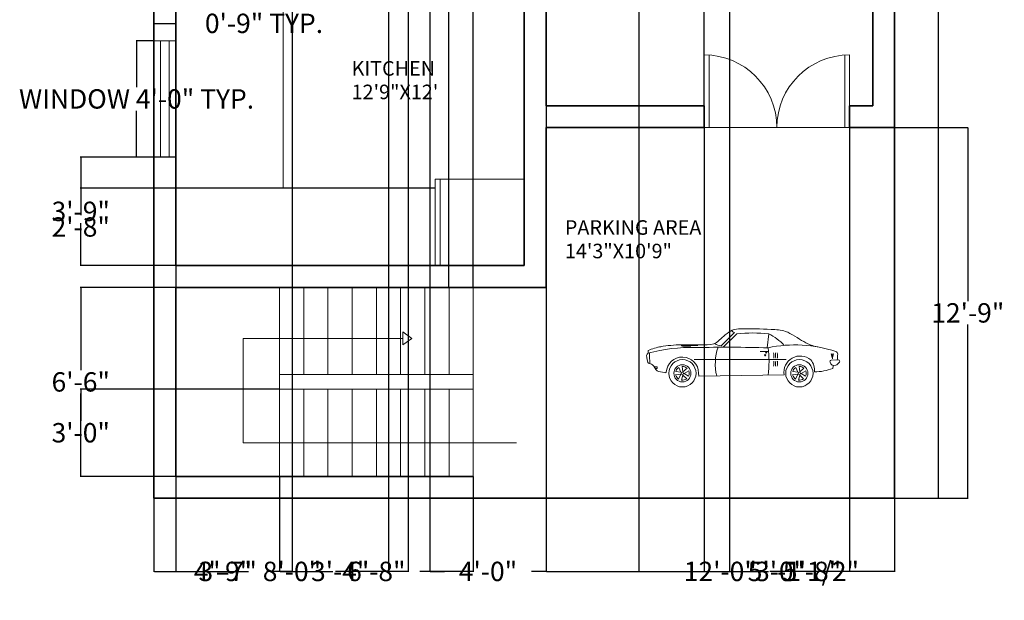
# Model space of a CAD drawing. Units: inches. Extents: x -69 to 405, y -4 to 680.
# Tile 1 of 3: x -34 to 372, y -4 to 236. Entities that reach past the tile are written whole.
import ezdxf

# ---------------------------------------------------------------- set-up
doc = ezdxf.new("R2010")
doc.units = ezdxf.units.IN
doc.header["$MEASUREMENT"] = 0
for name, color, linetype, lineweight in [('A-ANNO-DIMS', 4, 'Continuous', 18), ('A-AREA-IDEN', 4, 'Continuous', 18), ('A-EQPM-VEHI', 8, 'Continuous', 13), ('A-FLOR-CASE', 7, 'Continuous', 18), ('A-FLOR-STRS', 7, 'Continuous', 20), ('A-WALL', 7, 'Continuous', 35)]:
    doc.layers.add(name, color=color, linetype=linetype, lineweight=lineweight)
doc.layers.add('A-DOOR', color=2, linetype='Continuous', lineweight=18, true_color=0xf1eb1f)
doc.layers.add('A-GLAZ', color=85, linetype='Continuous', lineweight=18, true_color=0x58ba48)
doc.styles.get("Standard").update_dxf_attribs({"font": 'italic8.shx'})
doc.dimstyles.get("Standard").update_dxf_attribs({"dimtxt": 8, "dimasz": 0.18, "dimexe": 0.18, "dimexo": 0.0625, "dimgap": 0.09, "dimtad": 0, "dimtih": 1, "dimtoh": 1, "dimdec": 4, "dimzin": 0, "dimdsep": 46, "dimlunit": 3, "dimtxsty": 'Standard', "dimcen": 0.09, "dimadec": 0, "dimazin": 0, "dimtfac": 1, "dimtdec": 4, "dimtofl": 0, "dimtmove": 0, "dimatfit": 3, "dimfxl": 1, "dimtolj": 1, "dimtzin": 0, "dimarcsym": 0})

# ---------------------------------------------------------------- blocks, each defined once
blk = doc.blocks.new('*U2')
for p, q in [((72.93, 40.23), (85.8, 53.18)), ((75, 38.82), (88.08, 51.97)), ((119.39, 51.91), (117.92, 38.32)), ((50.13, 41.06), (34.31, 40.98)), ((43.26, 39.85), (35.15, 39.78)), ((35.3, 40.46), (50.13, 40.62)), ((111.09, 34.73), (118.48, 34.64)), ((7.45, 19.78), (9.74, 19.8)), ((46.65, 26.83), (136.29, 26.77)), ((179.3, 24.35), (180.25, 22.49)), ((180.37, 26.17), (187.51, 26.41)), ((182.62, 21.14), (184.91, 21.28)), ((186.68, 22.17), (188.51, 24.37)), ((9.76, 17.93), (8.53, 17.92)), ((10.37, 19.19), (10.38, 18.56)), ((50.87, 13.52), (50.91, 10.52))]:
    blk.add_line(p, q)
for points in [[(35.31, 39.93), (35.3, 40.27, 0.269532), (35.14, 40.54), (34.38, 40.96, 0.575383), (34.15, 40.83), (34.15, 40.49, 0.269532), (34.32, 40.22), (35.08, 39.79, 0.575383)], [(34.64, 20.05), (35.56, 14.97), (39.5, 18.31, 0.199906)], [(148.99, 20.05), (149.91, 14.97), (153.85, 18.31, 0.199906)], [(31.31, 7.72), (33.55, 12.37), (28.4, 11.99, 0.199906)], [(28.49, 15.1), (33.61, 14.4), (31.65, 19.18, 0.199906)], [(39.19, 8.12), (35.46, 11.69), (34.23, 6.67, 0.199906)], [(41.25, 15.74), (36.7, 13.3), (41.09, 10.58, 0.199906)], [(145.66, 7.72), (147.9, 12.37), (142.75, 11.99, 0.199906)], [(142.85, 15.1), (147.96, 14.4), (146.01, 19.18, 0.199906)], [(153.54, 8.12), (149.81, 11.69), (148.59, 6.67, 0.199906)], [(155.6, 15.74), (151.06, 13.3), (155.45, 10.58, 0.199906)]]:
    blk.add_lwpolyline(points, format="xyb", close=True)
for points in [[(181.58, 27.46), (181.53, 31.95), (180.48, 32.43)], [(181.58, 27.46), (181.53, 31.95), (182.57, 32.45)], [(50.91, 10.52), (134.38, 11.83)]]:
    blk.add_lwpolyline(points)
for centre, radius in [((115.89, 31.01), 0.619), ((34.98, 13.35), 13.35), ((34.98, 13.35), 8.35), ((149.33, 13.35), 13.35), ((149.33, 13.35), 8.35), ((34.98, 13.35), 1.25), ((149.33, 13.35), 1.25)]:
    blk.add_circle(centre, radius)
for centre, radius, start, end in [((114.6, 105.09), 59.37, 237.61027, 240.97846), ((103.45, -95), 147.78, 83.81633, 95.97054), ((95.51, 3.91), 53.61, 43.27479, 63.56652), ((42.18, -111.35), 149.91, 87.83928, 105.80965), ((20.53, -3.15), 43.06, 98.53035, 116.11198), ((80.1, -1364.13), 1402.96, 88.42296, 91.3179), ((73.29, 50.49), 10.26, 230.42401, 268.00854), ((118.31, 22.51), 51.16, 161.43071, 193.23633), ((145.17, -84.88), 125.99, 71.52833, 102.12419), ((79.16, 30.11), 76.3, 177.57734, 185.52052), ((34.98, 13.35), 15.9, 0.63732, 176.34123), ((25.66, 24.94), 94.01, 351.8279, 8.16738), ((45.64, 26.83), 78.76, 0.85201, 4.65562), ((47.43, 26.85), 78.76, 0.85201, 4.65562), ((49.23, 26.87), 78.76, 0.85201, 4.65562), ((150.1, 14.36), 15.92, 49.2263, 189.1528), ((216.26, 37.76), 36.17, 188.46832, 196.53145), ((146.68, 36.98), 36.17, 344.74319, 352.80633), ((184.3, 32.25), 2.49, 357.93203, 71.52833), ((116.55, 34.7), 70.29, 353.19423, 357.93203), ((9.75, 19.18), 0.623, 0.63732, 90.63732), ((45.64, 26.83), 78.76, 355.26443, 358.86328), ((47.43, 26.85), 78.76, 355.26443, 358.86328), ((49.23, 26.87), 78.76, 355.26443, 358.86328), ((149.4, 16.55), 14.84, 352.72855, 41.66131), ((180.41, 24.92), 1.25, 91.93898, 207.10902), ((182.47, 23.63), 2.49, 207.10902, 273.46767), ((114.25, 37.03), 70.29, 344.3985, 346.93849), ((184.76, 23.76), 2.49, 273.46767, 320.16835), ((187.55, 25.16), 1.25, 320.16835, 91.93898), ((9.76, 18.55), 0.623, 270.63732, 0.63732), ((162.47, 70.82), 56.18, 271.6865, 290.2774)]:
    blk.add_arc(centre, radius, start, end)
blk.add_ellipse((116.89, 33.59), major_axis=(-0.63, -0.007), ratio=0.610043)
for points, knots in [([(11.39, 38.92), (18.06, 40.19), (30.91, 42.01), (64.77, 40.11), (70.25, 44.91), (82.35, 56.38), (99.18, 57.3), (116.06, 56.35), (133.04, 55.87), (145.24, 49.87), (153.62, 43.8), (161.17, 40.68), (164.92, 39.73), (167.29, 39.15)], [18.629823, 18.629823, 18.629823, 18.629823, 19.527405, 20.700571, 21.107983, 21.608568, 21.92336, 23.151359, 23.716171, 23.908743, 24.77794, 24.943072, 25.187755, 25.187755, 25.187755, 25.187755]), ([(19.11, 14.36), (18.99, 14.21), (18.5, 13.81), (15.35, 15), (9.19, 13.94), (7.26, 22.22), (3.01, 22.66), (1.32, 23.61), (0.64, 26.92), (-0.96, 31.49), (1.54, 32.64), (1.5, 34.06), (1.49, 34.8), (1.49, 35.06), (1.52, 35.3), (1.58, 35.51)], [16.815853, 16.815853, 16.815853, 16.815853, 16.838212, 16.885395, 17.18439, 17.479846, 17.654423, 17.670693, 17.696923, 18.016358, 18.052739, 18.140805, 18.140805, 18.140805, 18.172382, 18.172382, 18.172382, 18.172382])]:
    blk.add_open_spline(points, degree=3, knots=knots)
blk = doc.blocks.new('*D5')
at = {"layer": 'A-ANNO-DIMS', "color": 0, "lineweight": -2, "transparency": 16777216}
for p, q in [((327.07, 638.28), (345.4, 638.28)), ((345.22, 638.1), (345.22, 343.14)), ((345.22, 38.46), (345.22, 333.43)), ((327.07, 38.28), (345.4, 38.28))]:
    blk.add_line(p, q, dxfattribs=at)
at = {"layer": 'A-ANNO-DIMS', "color": 0, "transparency": 16777216}
for points in [[(345.19, 638.1), (345.25, 638.1), (345.22, 638.28)], [(345.19, 38.46), (345.25, 38.46), (345.22, 38.28)]]:
    blk.add_solid(points, dxfattribs=at)
at = {"layer": 'Defpoints', "color": 0, "transparency": 16777216}
for p in [(327.01, 638.28), (327.01, 38.28), (345.22, 38.28)]:
    blk.add_point(p, dxfattribs=at)
at = {"layer": 'A-ANNO-DIMS', "color": 0, "transparency": 16777216, "insert": (345.22, 338.28), "char_height": 8, "attachment_point": 5}
blk.add_mtext("\\A1;50'", dxfattribs=at)
blk = doc.blocks.new('WIN-48IN')
for p, q in [((0, 48), (0, 0)), ((9, 48), (0, 48)), ((2.75, 48), (2.75, 0)), ((6.25, 48), (6.25, 0)), ((9, 0), (9, 48)), ((0, 0), (9, 0))]:
    blk.add_line(p, q)
blk = doc.blocks.new('*D16')
at = {"layer": 'A-ANNO-DIMS', "color": 0, "lineweight": -2, "transparency": 16777216}
for p, q in [((20.95, 227.12), (13.63, 227.12)), ((13.81, 226.94), (13.81, 207.97)), ((13.81, 179.3), (13.81, 198.26)), ((20.95, 179.12), (13.63, 179.12))]:
    blk.add_line(p, q, dxfattribs=at)
at = {"layer": 'A-ANNO-DIMS', "color": 0, "transparency": 16777216}
for points in [[(13.78, 226.94), (13.84, 226.94), (13.81, 227.12)], [(13.78, 179.3), (13.84, 179.3), (13.81, 179.12)]]:
    blk.add_solid(points, dxfattribs=at)
at = {"layer": 'Defpoints', "color": 0, "transparency": 16777216}
for p in [(13.81, 227.12), (21.01, 227.12), (21.01, 179.12)]:
    blk.add_point(p, dxfattribs=at)
at = {"layer": 'A-ANNO-DIMS', "color": 0, "transparency": 16777216, "insert": (13.81, 203.12), "char_height": 8, "attachment_point": 5}
blk.add_mtext('\\A1;WINDOW 4\'-0" TYP.', dxfattribs=at)
blk = doc.blocks.new('*D17')
at = {"layer": 'A-ANNO-DIMS', "color": 0, "lineweight": -2, "transparency": 16777216}
for p, q in [((21.01, 227.18), (21.01, 234.5)), ((21.19, 234.32), (29.83, 234.32)), ((30.01, 227.18), (30.01, 234.5)), ((30.01, 234.32), (30.19, 234.32))]:
    blk.add_line(p, q, dxfattribs=at)
at = {"layer": 'A-ANNO-DIMS', "color": 0, "transparency": 16777216}
for points in [[(21.19, 234.35), (21.19, 234.29), (21.01, 234.32)], [(29.83, 234.35), (29.83, 234.29), (30.01, 234.32)]]:
    blk.add_solid(points, dxfattribs=at)
at = {"layer": 'Defpoints', "color": 0, "transparency": 16777216}
for p in [(30.01, 234.32), (21.01, 227.12), (30.01, 227.12)]:
    blk.add_point(p, dxfattribs=at)
at = {"layer": 'A-ANNO-DIMS', "color": 0, "transparency": 16777216, "insert": (66.47, 234.32), "char_height": 8, "attachment_point": 5}
blk.add_mtext('\\A1;0\'-9" TYP.', dxfattribs=at)
blk = doc.blocks.new('*D24')
at = {"layer": 'A-ANNO-DIMS', "color": 0, "lineweight": -2, "transparency": 16777216}
for p, q in [((30.01, 47.22), (30.01, 7.85)), ((72.9, 47.22), (72.9, 7.85)), ((30.19, 8.03), (33.65, 8.03)), ((72.72, 8.03), (69.26, 8.03))]:
    blk.add_line(p, q, dxfattribs=at)
at = {"layer": 'A-ANNO-DIMS', "color": 0, "transparency": 16777216}
for points in [[(30.19, 8.06), (30.19, 8), (30.01, 8.03)], [(72.72, 8.06), (72.72, 8), (72.9, 8.03)]]:
    blk.add_solid(points, dxfattribs=at)
at = {"layer": 'Defpoints', "color": 0, "transparency": 16777216}
for p in [(30.01, 47.28), (72.9, 47.28), (72.9, 8.03)]:
    blk.add_point(p, dxfattribs=at)
at = {"layer": 'A-ANNO-DIMS', "color": 0, "transparency": 16777216, "insert": (51.46, 8.03), "char_height": 8, "attachment_point": 5}
blk.add_mtext('\\A1;3\'-7"', dxfattribs=at)
blk = doc.blocks.new('*D25')
at = {"layer": 'A-ANNO-DIMS', "color": 0, "lineweight": -2, "transparency": 16777216}
for p, q in [((72.9, 47.22), (72.9, 7.85)), ((152.9, 47.22), (152.9, 7.85)), ((73.08, 8.03), (94.91, 8.03)), ((152.72, 8.03), (130.9, 8.03))]:
    blk.add_line(p, q, dxfattribs=at)
at = {"layer": 'A-ANNO-DIMS', "color": 0, "transparency": 16777216}
for points in [[(73.08, 8.06), (73.08, 8), (72.9, 8.03)], [(152.72, 8.06), (152.72, 8), (152.9, 8.03)]]:
    blk.add_solid(points, dxfattribs=at)
at = {"layer": 'Defpoints', "color": 0, "transparency": 16777216}
for p in [(72.9, 47.28), (152.9, 47.28), (152.9, 8.03)]:
    blk.add_point(p, dxfattribs=at)
at = {"layer": 'A-ANNO-DIMS', "color": 0, "transparency": 16777216, "insert": (112.9, 8.03), "char_height": 8, "attachment_point": 5}
blk.add_mtext('\\A1;6\'-8"', dxfattribs=at)
blk = doc.blocks.new('*D26')
at = {"layer": 'A-ANNO-DIMS', "color": 0, "lineweight": -2, "transparency": 16777216}
for p, q in [((29.95, 125.28), (-9.42, 125.28)), ((-9.24, 125.1), (-9.24, 91.14)), ((-9.24, 47.46), (-9.24, 81.43)), ((29.95, 47.28), (-9.42, 47.28))]:
    blk.add_line(p, q, dxfattribs=at)
at = {"layer": 'A-ANNO-DIMS', "color": 0, "transparency": 16777216}
for points in [[(-9.27, 125.1), (-9.21, 125.1), (-9.24, 125.28)], [(-9.27, 47.46), (-9.21, 47.46), (-9.24, 47.28)]]:
    blk.add_solid(points, dxfattribs=at)
at = {"layer": 'Defpoints', "color": 0, "transparency": 16777216}
for p in [(-9.24, 125.28), (30.01, 125.28), (30.01, 47.28)]:
    blk.add_point(p, dxfattribs=at)
at = {"layer": 'A-ANNO-DIMS', "color": 0, "transparency": 16777216, "insert": (-9.24, 86.28), "char_height": 8, "attachment_point": 5}
blk.add_mtext('\\A1;6\'-6"', dxfattribs=at)
blk = doc.blocks.new('*D27')
at = {"layer": 'A-ANNO-DIMS', "color": 0, "lineweight": -2, "transparency": 16777216}
for p, q in [((72.84, 83.28), (-9.42, 83.28)), ((-9.24, 83.1), (-9.24, 70.14)), ((-9.24, 47.46), (-9.24, 60.43)), ((72.84, 47.28), (-9.42, 47.28))]:
    blk.add_line(p, q, dxfattribs=at)
at = {"layer": 'A-ANNO-DIMS', "color": 0, "transparency": 16777216}
for points in [[(-9.27, 83.1), (-9.21, 83.1), (-9.24, 83.28)], [(-9.27, 47.46), (-9.21, 47.46), (-9.24, 47.28)]]:
    blk.add_solid(points, dxfattribs=at)
at = {"layer": 'Defpoints', "color": 0, "transparency": 16777216}
for p in [(-9.24, 83.28), (72.9, 83.28), (72.9, 47.28)]:
    blk.add_point(p, dxfattribs=at)
at = {"layer": 'A-ANNO-DIMS', "color": 0, "transparency": 16777216, "insert": (-9.24, 65.28), "char_height": 8, "attachment_point": 5}
blk.add_mtext('\\A1;3\'-0"', dxfattribs=at)
blk = doc.blocks.new('*D28')
at = {"layer": 'A-ANNO-DIMS', "color": 0, "lineweight": -2, "transparency": 16777216}
for p, q in [((142.9, 125.35), (142.9, 668.71)), ((143.08, 668.53), (152.72, 668.53)), ((152.9, 125.35), (152.9, 668.71)), ((152.9, 668.53), (153.08, 668.53))]:
    blk.add_line(p, q, dxfattribs=at)
at = {"layer": 'A-ANNO-DIMS', "color": 0, "transparency": 16777216}
for points in [[(143.08, 668.56), (143.08, 668.5), (142.9, 668.53)], [(152.72, 668.56), (152.72, 668.5), (152.9, 668.53)]]:
    blk.add_solid(points, dxfattribs=at)
at = {"layer": 'Defpoints', "color": 0, "transparency": 16777216}
for p in [(152.9, 668.53), (142.9, 125.28), (152.9, 125.28)]:
    blk.add_point(p, dxfattribs=at)
at = {"layer": 'A-ANNO-DIMS', "color": 0, "transparency": 16777216, "insert": (173.75, 668.53), "char_height": 8, "attachment_point": 5}
blk.add_mtext('\\A1;0\'-10"', dxfattribs=at)
blk = doc.blocks.new('*D29')
at = {"layer": 'A-ANNO-DIMS', "color": 0, "lineweight": -2, "transparency": 16777216}
for p, q in [((183.01, 125.22), (183.01, 7.85)), ((327.01, 38.22), (327.01, 7.85)), ((183.19, 8.03), (234.54, 8.03)), ((326.83, 8.03), (275.48, 8.03))]:
    blk.add_line(p, q, dxfattribs=at)
at = {"layer": 'A-ANNO-DIMS', "color": 0, "transparency": 16777216}
for points in [[(183.19, 8.06), (183.19, 8), (183.01, 8.03)], [(326.83, 8.06), (326.83, 8), (327.01, 8.03)]]:
    blk.add_solid(points, dxfattribs=at)
at = {"layer": 'Defpoints', "color": 0, "transparency": 16777216}
for p in [(183.01, 125.28), (327.01, 38.28), (327.01, 8.03)]:
    blk.add_point(p, dxfattribs=at)
at = {"layer": 'A-ANNO-DIMS', "color": 0, "transparency": 16777216, "insert": (255.01, 8.03), "char_height": 8, "attachment_point": 5}
blk.add_mtext('\\A1;12\'-0"', dxfattribs=at)
blk = doc.blocks.new('*D30')
at = {"layer": 'A-ANNO-DIMS', "color": 0, "lineweight": -2, "transparency": 16777216}
for p, q in [((327.07, 191.28), (357.44, 191.28)), ((357.26, 191.1), (357.26, 119.64)), ((357.26, 38.46), (357.26, 109.93)), ((327.07, 38.28), (357.44, 38.28))]:
    blk.add_line(p, q, dxfattribs=at)
at = {"layer": 'A-ANNO-DIMS', "color": 0, "transparency": 16777216}
for points in [[(357.23, 191.1), (357.29, 191.1), (357.26, 191.28)], [(357.23, 38.46), (357.29, 38.46), (357.26, 38.28)]]:
    blk.add_solid(points, dxfattribs=at)
at = {"layer": 'Defpoints', "color": 0, "transparency": 16777216}
for p in [(327.01, 191.28), (327.01, 38.28), (357.26, 38.28)]:
    blk.add_point(p, dxfattribs=at)
at = {"layer": 'A-ANNO-DIMS', "color": 0, "transparency": 16777216, "insert": (357.26, 114.78), "char_height": 8, "attachment_point": 5}
blk.add_mtext('\\A1;12\'-9"', dxfattribs=at)
blk = doc.blocks.new('*D31')
at = {"layer": 'A-ANNO-DIMS', "color": 0, "lineweight": -2, "transparency": 16777216}
for p, q in [((248.38, 191.22), (248.38, 7.85)), ((308.38, 191.22), (308.38, 7.85)), ((248.56, 8.03), (260.39, 8.03)), ((308.2, 8.03), (296.38, 8.03))]:
    blk.add_line(p, q, dxfattribs=at)
at = {"layer": 'A-ANNO-DIMS', "color": 0, "transparency": 16777216}
for points in [[(248.56, 8.06), (248.56, 8), (248.38, 8.03)], [(308.2, 8.06), (308.2, 8), (308.38, 8.03)]]:
    blk.add_solid(points, dxfattribs=at)
at = {"layer": 'Defpoints', "color": 0, "transparency": 16777216}
for p in [(248.38, 191.28), (308.38, 191.28), (308.38, 8.03)]:
    blk.add_point(p, dxfattribs=at)
at = {"layer": 'A-ANNO-DIMS', "color": 0, "transparency": 16777216, "insert": (278.38, 8.03), "char_height": 8, "attachment_point": 5}
blk.add_mtext('\\A1;5\'-0"', dxfattribs=at)
blk = doc.blocks.new('*D32')
at = {"layer": 'A-ANNO-DIMS', "color": 0, "lineweight": -2, "transparency": 16777216}
for p, q in [((183.01, 200.35), (183.01, 668.71)), ((183.19, 668.53), (248.2, 668.53)), ((248.38, 200.35), (248.38, 668.71)), ((248.38, 668.53), (248.56, 668.53))]:
    blk.add_line(p, q, dxfattribs=at)
at = {"layer": 'A-ANNO-DIMS', "color": 0, "transparency": 16777216}
for points in [[(183.19, 668.56), (183.19, 668.5), (183.01, 668.53)], [(248.2, 668.56), (248.2, 668.5), (248.38, 668.53)]]:
    blk.add_solid(points, dxfattribs=at)
at = {"layer": 'Defpoints', "color": 0, "transparency": 16777216}
for p in [(248.38, 668.53), (183.01, 200.28), (248.38, 200.28)]:
    blk.add_point(p, dxfattribs=at)
at = {"layer": 'A-ANNO-DIMS', "color": 0, "transparency": 16777216, "insert": (281.8, 668.53), "char_height": 8, "attachment_point": 5}
blk.add_mtext('\\A1;5\'-5 1/2"', dxfattribs=at)
blk = doc.blocks.new('*D33')
at = {"layer": 'A-ANNO-DIMS', "color": 0, "lineweight": -2, "transparency": 16777216}
for p, q in [((30.01, 350.22), (30.01, 7.85)), ((126.01, 350.22), (126.01, 7.85)), ((30.19, 8.03), (60.01, 8.03)), ((125.83, 8.03), (96, 8.03))]:
    blk.add_line(p, q, dxfattribs=at)
at = {"layer": 'A-ANNO-DIMS', "color": 0, "transparency": 16777216}
for points in [[(30.19, 8.06), (30.19, 8), (30.01, 8.03)], [(125.83, 8.06), (125.83, 8), (126.01, 8.03)]]:
    blk.add_solid(points, dxfattribs=at)
at = {"layer": 'Defpoints', "color": 0, "transparency": 16777216}
for p in [(30.01, 350.28), (126.01, 350.28), (126.01, 8.03)]:
    blk.add_point(p, dxfattribs=at)
at = {"layer": 'A-ANNO-DIMS', "color": 0, "transparency": 16777216, "insert": (78.01, 8.03), "char_height": 8, "attachment_point": 5}
blk.add_mtext('\\A1;8\'-0"', dxfattribs=at)
blk = doc.blocks.new('*D40')
at = {"layer": 'A-ANNO-DIMS', "color": 0, "lineweight": -2, "transparency": 16777216}
for p, q in [((135.01, 407.22), (135.01, 7.85)), ((183.01, 407.22), (183.01, 7.85)), ((135.19, 8.03), (141.01, 8.03)), ((182.83, 8.03), (177, 8.03))]:
    blk.add_line(p, q, dxfattribs=at)
at = {"layer": 'A-ANNO-DIMS', "color": 0, "transparency": 16777216}
for points in [[(135.19, 8.06), (135.19, 8), (135.01, 8.03)], [(182.83, 8.06), (182.83, 8), (183.01, 8.03)]]:
    blk.add_solid(points, dxfattribs=at)
at = {"layer": 'Defpoints', "color": 0, "transparency": 16777216}
for p in [(135.01, 407.28), (183.01, 407.28), (183.01, 8.03)]:
    blk.add_point(p, dxfattribs=at)
at = {"layer": 'A-ANNO-DIMS', "color": 0, "transparency": 16777216, "insert": (159.01, 8.03), "char_height": 8, "attachment_point": 5}
blk.add_mtext('\\A1;4\'-0"', dxfattribs=at)
blk = doc.blocks.new('*D44')
at = {"layer": 'A-ANNO-DIMS', "color": 0, "lineweight": -2, "transparency": 16777216}
for p, q in [((21.01, 638.22), (21.01, 7.85)), ((78.06, 638.22), (78.06, 7.85)), ((21.19, 8.03), (31.54, 8.03)), ((77.88, 8.03), (67.53, 8.03))]:
    blk.add_line(p, q, dxfattribs=at)
at = {"layer": 'A-ANNO-DIMS', "color": 0, "transparency": 16777216}
for points in [[(21.19, 8.06), (21.19, 8), (21.01, 8.03)], [(77.88, 8.06), (77.88, 8), (78.06, 8.03)]]:
    blk.add_solid(points, dxfattribs=at)
at = {"layer": 'Defpoints', "color": 0, "transparency": 16777216}
for p in [(21.01, 638.28), (78.06, 638.28), (78.06, 8.03)]:
    blk.add_point(p, dxfattribs=at)
at = {"layer": 'A-ANNO-DIMS', "color": 0, "transparency": 16777216, "insert": (49.53, 8.03), "char_height": 8, "attachment_point": 5}
blk.add_mtext('\\A1;4\'-9"', dxfattribs=at)
blk = doc.blocks.new('*D45')
at = {"layer": 'A-ANNO-DIMS', "color": 0, "lineweight": -2, "transparency": 16777216}
for p, q in [((78.06, 638.22), (78.06, 7.85)), ((117.87, 638.22), (117.87, 7.85)), ((78.24, 8.03), (79.97, 8.03)), ((117.69, 8.03), (115.96, 8.03))]:
    blk.add_line(p, q, dxfattribs=at)
at = {"layer": 'A-ANNO-DIMS', "color": 0, "transparency": 16777216}
for points in [[(78.24, 8.06), (78.24, 8), (78.06, 8.03)], [(117.69, 8.06), (117.69, 8), (117.87, 8.03)]]:
    blk.add_solid(points, dxfattribs=at)
at = {"layer": 'Defpoints', "color": 0, "transparency": 16777216}
for p in [(78.06, 638.28), (117.87, 638.28), (117.87, 8.03)]:
    blk.add_point(p, dxfattribs=at)
at = {"layer": 'A-ANNO-DIMS', "color": 0, "transparency": 16777216, "insert": (97.96, 8.03), "char_height": 8, "attachment_point": 5}
blk.add_mtext('\\A1;3\'-4"', dxfattribs=at)
blk = doc.blocks.new('*D46')
at = {"layer": 'A-ANNO-DIMS', "color": 0, "lineweight": -2, "transparency": 16777216}
for p, q in [((221.33, 638.22), (221.33, 7.85)), ((258.77, 638.22), (258.77, 7.85)), ((221.51, 8.03), (258.59, 8.03)), ((258.77, 8.03), (258.95, 8.03))]:
    blk.add_line(p, q, dxfattribs=at)
at = {"layer": 'A-ANNO-DIMS', "color": 0, "transparency": 16777216}
for points in [[(221.51, 8.06), (221.51, 8), (221.33, 8.03)], [(258.59, 8.06), (258.59, 8), (258.77, 8.03)]]:
    blk.add_solid(points, dxfattribs=at)
at = {"layer": 'Defpoints', "color": 0, "transparency": 16777216}
for p in [(221.33, 638.28), (258.77, 638.28), (258.77, 8.03)]:
    blk.add_point(p, dxfattribs=at)
at = {"layer": 'A-ANNO-DIMS', "color": 0, "transparency": 16777216, "insert": (290.85, 8.03), "char_height": 8, "attachment_point": 5}
blk.add_mtext('\\A1;3\'-1 1/2"', dxfattribs=at)
blk = doc.blocks.new('*D47')
at = {"layer": 'A-ANNO-DIMS', "color": 0, "lineweight": -2, "transparency": 16777216}
for p, q in [((258.77, 638.22), (258.77, 7.85)), ((327.01, 638.22), (327.01, 7.85)), ((258.95, 8.03), (274.89, 8.03)), ((326.83, 8.03), (310.88, 8.03))]:
    blk.add_line(p, q, dxfattribs=at)
at = {"layer": 'A-ANNO-DIMS', "color": 0, "transparency": 16777216}
for points in [[(258.95, 8.06), (258.95, 8), (258.77, 8.03)], [(326.83, 8.06), (326.83, 8), (327.01, 8.03)]]:
    blk.add_solid(points, dxfattribs=at)
at = {"layer": 'Defpoints', "color": 0, "transparency": 16777216}
for p in [(258.77, 638.28), (327.01, 638.28), (327.01, 8.03)]:
    blk.add_point(p, dxfattribs=at)
at = {"layer": 'A-ANNO-DIMS', "color": 0, "transparency": 16777216, "insert": (292.89, 8.03), "char_height": 8, "attachment_point": 5}
blk.add_mtext('\\A1;5\'-8"', dxfattribs=at)
blk = doc.blocks.new('*D50')
at = {"layer": 'A-ANNO-DIMS', "color": 0, "lineweight": -2, "transparency": 16777216}
for p, q in [((29.95, 179.12), (-9.42, 179.12)), ((-9.24, 178.94), (-9.24, 161.55)), ((-9.24, 134.46), (-9.24, 151.85)), ((29.95, 134.28), (-9.42, 134.28))]:
    blk.add_line(p, q, dxfattribs=at)
at = {"layer": 'A-ANNO-DIMS', "color": 0, "transparency": 16777216}
for points in [[(-9.27, 178.94), (-9.21, 178.94), (-9.24, 179.12)], [(-9.27, 134.46), (-9.21, 134.46), (-9.24, 134.28)]]:
    blk.add_solid(points, dxfattribs=at)
at = {"layer": 'Defpoints', "color": 0, "transparency": 16777216}
for p in [(-9.24, 179.12), (30.01, 179.12), (30.01, 134.28)]:
    blk.add_point(p, dxfattribs=at)
at = {"layer": 'A-ANNO-DIMS', "color": 0, "transparency": 16777216, "insert": (-9.24, 156.7), "char_height": 8, "attachment_point": 5}
blk.add_mtext('\\A1;3\'-9"', dxfattribs=at)
blk = doc.blocks.new('*D64')
at = {"layer": 'A-ANNO-DIMS', "color": 0, "lineweight": -2, "transparency": 16777216}
for p, q in [((137.12, 166.22), (-9.42, 166.22)), ((-9.24, 166.04), (-9.24, 155.11)), ((-9.24, 134.46), (-9.24, 145.4)), ((137.12, 134.28), (-9.42, 134.28))]:
    blk.add_line(p, q, dxfattribs=at)
at = {"layer": 'A-ANNO-DIMS', "color": 0, "transparency": 16777216}
for points in [[(-9.27, 166.04), (-9.21, 166.04), (-9.24, 166.22)], [(-9.27, 134.46), (-9.21, 134.46), (-9.24, 134.28)]]:
    blk.add_solid(points, dxfattribs=at)
at = {"layer": 'Defpoints', "color": 0, "transparency": 16777216}
for p in [(-9.24, 166.22), (137.19, 166.22), (137.19, 134.28)]:
    blk.add_point(p, dxfattribs=at)
at = {"layer": 'A-ANNO-DIMS', "color": 0, "transparency": 16777216, "insert": (-9.24, 150.25), "char_height": 8, "attachment_point": 5}
blk.add_mtext('\\A1;2\'-8"', dxfattribs=at)

msp = doc.modelspace()

# ---------------------------------------------------------------- linework, layer by layer
at = {"layer": 'A-DOOR'}
for p, q in [((248.38397, 191.28441), (248.38397, 221.28441)), ((250.38397, 191.28441), (250.38397, 221.21767)), ((306.38397, 191.28441), (306.38397, 221.21767)), ((308.38397, 191.28441), (308.38397, 221.28441)), ((248.38397, 191.28441), (308.38397, 191.28441))]:
    msp.add_line(p, q, dxfattribs=at)
for centre, start, end in [((248.38397, 191.28441), 0, 90), ((308.38397, 191.28441), 90, 180)]:
    msp.add_arc(centre, 30, start, end, dxfattribs=at)
at = {"layer": 'A-FLOR-CASE'}
for p, q in [((74.39466, 278.28441), (74.39466, 166.22496)), ((137.18616, 169.94012), (174.00851, 169.94012)), ((137.18616, 169.94012), (137.18616, 134.28441)), ((139.18616, 169.94012), (139.18616, 134.28441)), ((74.39466, 166.22496), (137.18616, 166.22496))]:
    msp.add_line(p, q, dxfattribs=at)
at = {"layer": 'A-FLOR-STRS'}
for p, q in [((72.90475, 47.28441), (72.90475, 125.28441)), ((82.90475, 89.28441), (82.90475, 125.28441)), ((92.90475, 89.28441), (92.90475, 125.28441)), ((102.90475, 89.28441), (102.90475, 125.28441)), ((112.90475, 89.28441), (112.90475, 125.28441)), ((122.90475, 89.28441), (122.90475, 125.28441)), ((132.90475, 89.28441), (132.90475, 125.28441)), ((142.90475, 89.28441), (142.90475, 125.28441)), ((152.90475, 125.28441), (152.90475, 38.28441)), ((123.8929, 106.90219), (127.59229, 104.25616)), ((123.8929, 106.90219), (123.8929, 101.61013)), ((57.81404, 61.0962), (57.81404, 104.25616)), ((57.81404, 104.25616), (123.8929, 104.25616)), ((123.8929, 101.61013), (127.59229, 104.25616)), ((72.90475, 89.28441), (152.90475, 89.28441)), ((72.90475, 83.28441), (152.90475, 83.28441)), ((82.90475, 47.28441), (82.90475, 83.28441)), ((92.90475, 47.28441), (92.90475, 83.28441)), ((102.90475, 47.28441), (102.90475, 83.28441)), ((112.90475, 47.28441), (112.90475, 83.28441)), ((122.90475, 47.28441), (122.90475, 83.28441)), ((132.90475, 47.28441), (132.90475, 83.28441)), ((142.90475, 47.28441), (142.90475, 83.28441)), ((170.77819, 61.0962), (57.81404, 61.0962))]:
    msp.add_line(p, q, dxfattribs=at)
at = {"layer": 'A-WALL'}
for p, q in [((183.00851, 407.28441), (183.00851, 200.28441)), ((318.00851, 200.28441), (318.00851, 398.28441)), ((174.00851, 370.08876), (174.00851, 134.28441)), ((30.00851, 278.28441), (30.00851, 134.28441)), ((248.38397, 200.28441), (183.00851, 200.28441)), ((248.38397, 191.28441), (248.38397, 200.28441)), ((318.00851, 200.28441), (308.38397, 200.28441)), ((308.38397, 191.28441), (308.38397, 200.28441)), ((183.00851, 191.28441), (183.00851, 125.28441)), ((248.38397, 191.28441), (183.00851, 191.28441)), ((327.00851, 191.28441), (308.38397, 191.28441)), ((30.00851, 134.28441), (174.00851, 134.28441)), ((30.00851, 125.28441), (183.00851, 125.28441)), ((30.00851, 125.28441), (30.00851, 47.28441)), ((30.00851, 47.28441), (152.90475, 47.28441))]:
    msp.add_line(p, q, dxfattribs=at)
msp.add_lwpolyline([(21.00851, 38.28441), (327.00851, 38.28441), (327.00851, 638.28441), (21.00851, 638.28441)], close=True, dxfattribs=at)

# ---------------------------------------------------------------- block references
at = {"layer": 'A-EQPM-VEHI', "xscale": 0.4226362095738097, "yscale": 0.4226362095738097, "zscale": 0.4226362095738097}
msp.add_blockref('*U2', (224.54904, 84.17506), dxfattribs=at)
at = {"layer": 'A-GLAZ'}
msp.add_blockref('WIN-48IN', (21.00851, 179.11596), dxfattribs=at)

# ---------------------------------------------------------------- texts
at = {"layer": 'A-AREA-IDEN'}
for s, p in [('KITCHEN', (102.65617, 212.72563)), ('12\'9"X12\'', (102.65617, 203.01135)), ('PARKING AREA', (190.76919, 147.03298)), ('14\'3"X10\'9"', (190.76919, 137.31869))]:
    msp.add_text(s, height=6, dxfattribs=at).set_placement(p)

# ---------------------------------------------------------------- dimensions: what is measured, and where the dimension line sits
at = {"layer": 'A-ANNO-DIMS'}
for base, p1, p2, picture, middle in [((248.38397, 668.53441), (183.00851, 200.28441), (248.38397, 200.28441), '*D32', (281.79683, 668.53441)), ((152.90475, 668.53441), (142.90475, 125.28441), (152.90475, 125.28441), '*D28', (173.74618, 668.53441)), ((78.0556, 8.03441), (21.00851, 638.28441), (78.0556, 638.28441), '*D44', (49.53205, 8.03441)), ((117.8737, 8.03441), (78.0556, 638.28441), (117.8737, 638.28441), '*D45', (97.96465, 8.03441)), ((258.76903, 8.03441), (221.3312, 638.28441), (258.76903, 638.28441), '*D46', (290.84856, 8.03441)), ((327.00851, 8.03441), (258.76903, 638.28441), (327.00851, 638.28441), '*D47', (292.88877, 8.03441)), ((183.00851, 8.03441), (135.00851, 407.28441), (183.00851, 407.28441), '*D40', (159.00851, 8.03441)), ((126.00851, 8.03441), (30.00851, 350.28441), (126.00851, 350.28441), '*D33', (78.00851, 8.03441)), ((308.38397, 8.03441), (248.38397, 191.28441), (308.38397, 191.28441), '*D31', (278.38397, 8.03441)), ((327.00851, 8.03441), (183.00851, 125.28441), (327.00851, 38.28441), '*D29', (255.00851, 8.03441)), ((72.90475, 8.03441), (30.00851, 47.28441), (72.90475, 47.28441), '*D24', (51.45663, 8.03441)), ((152.90475, 8.03441), (72.90475, 47.28441), (152.90475, 47.28441), '*D25', (112.90475, 8.03441))]:
    dim = msp.add_linear_dim(base=base, p1=p1, p2=p2, dimstyle='Standard', override={"dimdec": 1, "dimlfac": 1, "dimrnd": 0, "dimzin": 1, "dimdsep": 46, "dimlunit": 4, "dimfrac": 2}, dxfattribs=at)
    dim.commit()
    dim.dimension.update_dxf_attribs({"geometry": picture, "text_midpoint": middle})
for base, p1, p2, override, picture, middle in [((345.22225, 38.28441), (327.00851, 638.28441), (327.00851, 38.28441), {"dimclrd": 0, "dimclre": 0, "dimclrt": 0}, '*D5', (345.22225, 338.28441)), ((357.25851, 38.28441), (327.00851, 191.28441), (327.00851, 38.28441), {"dimdec": 1, "dimlfac": 1, "dimrnd": 0, "dimzin": 1, "dimdsep": 46, "dimlunit": 4, "dimfrac": 2}, '*D30', (357.25851, 114.78441)), ((-9.24149, 179.11596), (30.00851, 134.28441), (30.00851, 179.11596), {"dimdec": 1, "dimlfac": 1, "dimrnd": 0, "dimzin": 1, "dimdsep": 46, "dimlunit": 4, "dimfrac": 2}, '*D50', (-9.24149, 156.70018)), ((-9.24149, 166.22496), (137.18616, 134.28441), (137.18616, 166.22496), {"dimdec": 1, "dimlfac": 1, "dimrnd": 0, "dimzin": 1, "dimdsep": 46, "dimlunit": 4, "dimfrac": 2}, '*D64', (-9.24149, 150.25468)), ((-9.24149, 125.28441), (30.00851, 47.28441), (30.00851, 125.28441), {"dimdec": 1, "dimlfac": 1, "dimrnd": 0, "dimzin": 1, "dimdsep": 46, "dimlunit": 4, "dimfrac": 2}, '*D26', (-9.24149, 86.28441)), ((-9.24149, 83.28441), (72.90475, 47.28441), (72.90475, 83.28441), {"dimdec": 1, "dimlfac": 1, "dimrnd": 0, "dimzin": 1, "dimdsep": 46, "dimlunit": 4, "dimfrac": 2}, '*D27', (-9.24149, 65.28441))]:
    dim = msp.add_linear_dim(base=base, p1=p1, p2=p2, angle=90, dimstyle='Standard', override=override, dxfattribs=at)
    dim.commit()
    dim.dimension.update_dxf_attribs({"geometry": picture, "text_midpoint": middle})
dim = msp.add_linear_dim(base=(30.00851, 234.31596), p1=(21.00851, 227.11596), p2=(30.00851, 227.11596), text='<> TYP.', dimstyle='Standard', override={"dimdec": 1, "dimlfac": 1, "dimrnd": 0, "dimzin": 1, "dimdsep": 46, "dimlunit": 4, "dimfrac": 2}, dxfattribs=at)
dim.commit()
dim.dimension.update_dxf_attribs({"geometry": '*D17', "text_midpoint": (66.46899, 234.31596)})
dim = msp.add_linear_dim(base=(13.80851, 227.11596), p1=(21.00851, 179.11596), p2=(21.00851, 227.11596), angle=90, text='WINDOW <> TYP.', dimstyle='Standard', override={"dimdec": 1, "dimlfac": 1, "dimrnd": 0, "dimzin": 1, "dimdsep": 46, "dimlunit": 4, "dimfrac": 2}, dxfattribs=at)
dim.commit()
dim.dimension.update_dxf_attribs({"geometry": '*D16', "text_midpoint": (13.80851, 203.11596)})

doc.saveas('drawing.dxf')
